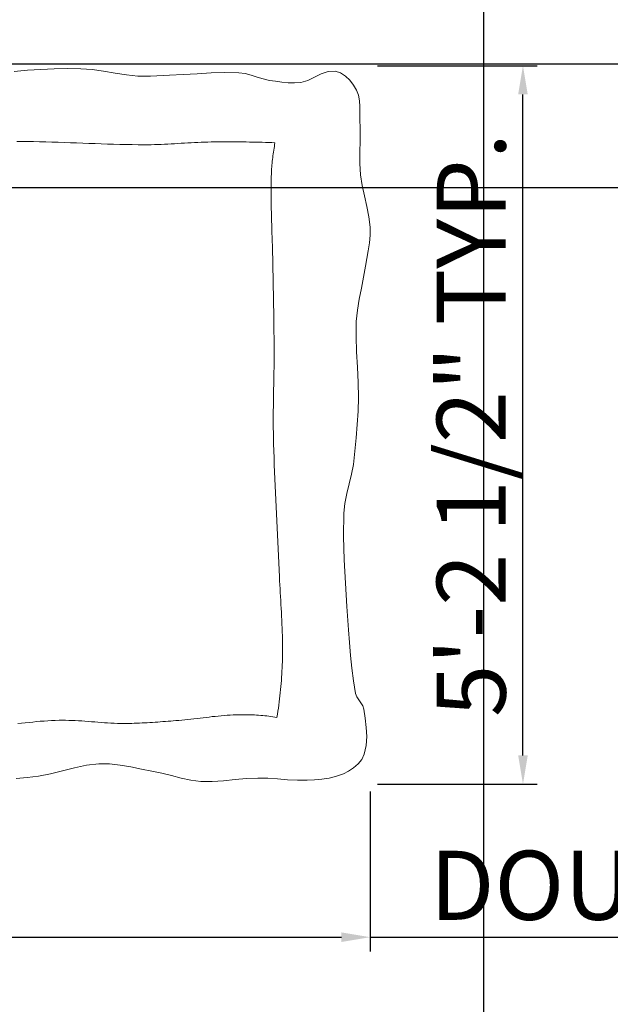
# Model space of a CAD drawing. Units: inches. Extents: x 2656 to 9931, y 1941 to 3068.
# Tile 12 of 46: x 2811 to 2863, y 2484 to 2569. Entities that reach past the tile are written whole.
import ezdxf

# ---------------------------------------------------------------- set-up
doc = ezdxf.new("R2010")
doc.units = ezdxf.units.IN
doc.layers.add('A-ANNO-DIMS', color=2, linetype='Continuous', lineweight=18)
doc.layers.add('A-FURN', color=8, linetype='Continuous', lineweight=13)
doc.styles.get("Standard").update_dxf_attribs({"font": 'arial.ttf'})
doc.dimstyles.new('ISO-25', dxfattribs={"dimtxt": 6, "dimasz": 2.5, "dimexe": 1.25, "dimexo": 0.625, "dimtad": 1, "dimdec": 0, "dimlunit": 3, "dimtxsty": 'Standard', "dimcen": 2.5, "dimadec": 0, "dimazin": 0, "dimtfac": 1, "dimtdec": 0, "dimtmove": 0, "dimatfit": 3, "dimfxl": 1, "dimarcsym": 0})

# ---------------------------------------------------------------- blocks, each defined once
blk = doc.blocks.new('BED-DOUBLE')
for p, q in [((58.764, 62.009), (57.607, 61.902)), ((59.923, 62.092), (58.764, 62.009)), ((61.084, 62.147), (59.923, 62.092)), ((62.246, 62.166), (61.084, 62.147)), ((63.407, 62.146), (62.246, 62.166)), ((64.403, 62.069), (63.407, 62.146)), ((65.395, 61.932), (64.403, 62.069)), ((66.384, 61.77), (65.395, 61.932)), ((67.375, 61.618), (66.384, 61.77)), ((68.37, 61.511), (67.375, 61.618)), ((72.325, 61.635), (71.116, 61.578)), ((73.533, 61.711), (72.325, 61.635)), ((74.742, 61.781), (73.533, 61.711)), ((75.95, 61.817), (74.742, 61.781)), ((77.158, 61.794), (75.95, 61.817)), ((77.698, 61.721), (77.158, 61.794)), ((78.229, 61.583), (77.698, 61.721)), ((84.331, 61.693), (83.743, 61.407)), ((84.926, 61.898), (84.331, 61.693)), ((85.537, 61.929), (84.926, 61.898)), ((86.008, 61.785), (85.537, 61.929)), ((86.434, 61.514), (86.008, 61.785)), ((68.918, 61.489), (68.37, 61.511)), ((69.467, 61.497), (68.918, 61.489)), ((70.017, 61.522), (69.467, 61.497)), ((70.567, 61.553), (70.017, 61.522)), ((71.116, 61.578), (70.567, 61.553)), ((78.755, 61.415), (78.229, 61.583)), ((79.283, 61.255), (78.755, 61.415)), ((79.819, 61.137), (79.283, 61.255)), ((80.36, 61.054), (79.819, 61.137)), ((80.905, 60.98), (80.36, 61.054)), ((81.45, 60.93), (80.905, 60.98)), ((81.996, 60.92), (81.45, 60.93)), ((82.537, 60.963), (81.996, 60.92)), ((83.149, 61.132), (82.537, 60.963)), ((83.743, 61.407), (83.149, 61.132)), ((86.811, 61.15), (86.434, 61.514)), ((87.134, 60.731), (86.811, 61.15)), ((87.398, 60.291), (87.134, 60.731)), ((87.572, 59.839), (87.398, 60.291)), ((87.658, 59.358), (87.572, 59.839)), ((87.686, 58.86), (87.658, 59.358)), ((87.688, 58.356), (87.686, 58.86)), ((87.698, 57.859), (87.688, 58.356)), ((87.718, 56.87), (87.698, 57.859)), ((87.706, 55.879), (87.718, 56.87)), ((58.21, 55.827), (57.849, 55.828)), ((58.746, 55.822), (58.21, 55.827)), ((59.283, 55.814), (58.746, 55.822)), ((59.819, 55.803), (59.283, 55.814)), ((60.355, 55.789), (59.819, 55.803)), ((60.892, 55.774), (60.355, 55.789)), ((61.428, 55.756), (60.892, 55.774)), ((61.964, 55.738), (61.428, 55.756)), ((62.5, 55.718), (61.964, 55.738)), ((63.037, 55.698), (62.5, 55.718)), ((63.573, 55.678), (63.037, 55.698)), ((64.109, 55.657), (63.573, 55.678)), ((64.645, 55.638), (64.109, 55.657)), ((65.181, 55.619), (64.645, 55.638)), ((65.718, 55.601), (65.181, 55.619)), ((71.546, 55.63), (71.256, 55.614)), ((71.836, 55.648), (71.546, 55.63)), ((72.126, 55.665), (71.836, 55.648)), ((72.416, 55.682), (72.126, 55.665)), ((72.706, 55.7), (72.416, 55.682)), ((72.996, 55.716), (72.706, 55.7)), ((73.286, 55.731), (72.996, 55.716)), ((73.576, 55.745), (73.286, 55.731)), ((73.866, 55.758), (73.576, 55.745)), ((74.156, 55.769), (73.866, 55.758)), ((74.446, 55.777), (74.156, 55.769)), ((74.736, 55.783), (74.446, 55.777)), ((75.014, 55.787), (74.736, 55.783)), ((75.293, 55.79), (75.014, 55.787)), ((75.571, 55.792), (75.293, 55.79)), ((75.85, 55.793), (75.571, 55.792)), ((76.128, 55.794), (75.85, 55.793)), ((76.406, 55.794), (76.128, 55.794)), ((76.685, 55.793), (76.406, 55.794)), ((76.963, 55.792), (76.685, 55.793)), ((77.242, 55.789), (76.963, 55.792)), ((77.52, 55.786), (77.242, 55.789)), ((77.799, 55.782), (77.52, 55.786)), ((78.077, 55.778), (77.799, 55.782)), ((78.355, 55.772), (78.077, 55.778)), ((78.634, 55.766), (78.355, 55.772)), ((78.912, 55.759), (78.634, 55.766)), ((79.19, 55.751), (78.912, 55.759)), ((79.469, 55.743), (79.19, 55.751)), ((79.747, 55.733), (79.469, 55.743)), ((80.025, 55.723), (79.747, 55.733)), ((80.303, 55.712), (80.025, 55.723)), ((80.274, 55.552), (80.303, 55.712)), ((87.688, 54.889), (87.706, 55.879)), ((66.254, 55.584), (65.718, 55.601)), ((66.79, 55.57), (66.254, 55.584)), ((67.327, 55.558), (66.79, 55.57)), ((67.863, 55.548), (67.327, 55.558)), ((68.399, 55.542), (67.863, 55.548)), ((68.936, 55.538), (68.399, 55.542)), ((69.226, 55.539), (68.936, 55.538)), ((69.516, 55.543), (69.226, 55.539)), ((69.806, 55.55), (69.516, 55.543)), ((70.096, 55.559), (69.806, 55.55)), ((70.386, 55.57), (70.096, 55.559)), ((70.676, 55.583), (70.386, 55.57)), ((70.966, 55.598), (70.676, 55.583)), ((71.256, 55.614), (70.966, 55.598)), ((80.146, 54.748), (80.169, 54.909)), ((80.169, 54.909), (80.193, 55.07)), ((80.193, 55.07), (80.219, 55.231)), ((80.219, 55.231), (80.246, 55.392)), ((80.246, 55.392), (80.274, 55.552)), ((87.693, 53.9), (87.688, 54.889)), ((80.038, 53.776), (80.053, 53.938)), ((80.053, 53.938), (80.069, 54.1)), ((80.069, 54.1), (80.086, 54.262)), ((80.086, 54.262), (80.105, 54.424)), ((80.105, 54.424), (80.125, 54.586)), ((80.125, 54.586), (80.146, 54.748)), ((79.985, 52.963), (79.993, 53.125)), ((79.993, 53.125), (80.002, 53.288)), ((80.002, 53.288), (80.013, 53.451)), ((80.013, 53.451), (80.025, 53.613)), ((80.025, 53.613), (80.038, 53.776)), ((87.749, 52.913), (87.693, 53.9)), ((79.965, 52.119), (79.97, 52.475)), ((79.97, 52.475), (79.974, 52.637)), ((79.974, 52.637), (79.979, 52.8)), ((79.979, 52.8), (79.985, 52.963)), ((87.883, 51.998), (87.749, 52.913)), ((79.962, 51.764), (79.965, 52.119)), ((79.962, 51.408), (79.962, 51.764)), ((79.963, 51.053), (79.962, 51.408)), ((88.08, 51.092), (87.883, 51.998)), ((79.967, 50.698), (79.963, 51.053)), ((79.972, 50.342), (79.967, 50.698)), ((88.293, 50.188), (88.08, 51.092)), ((79.979, 49.987), (79.972, 50.342)), ((79.988, 49.631), (79.979, 49.987)), ((79.997, 49.276), (79.988, 49.631)), ((88.476, 49.281), (88.293, 50.188)), ((80.007, 48.921), (79.997, 49.276)), ((80.018, 48.565), (80.007, 48.921)), ((88.582, 48.364), (88.476, 49.281)), ((80.029, 48.21), (80.018, 48.565)), ((80.041, 47.854), (80.029, 48.21)), ((88.58, 47.686), (88.582, 48.364)), ((80.052, 47.499), (80.041, 47.854)), ((80.063, 47.143), (80.052, 47.499)), ((80.074, 46.788), (80.063, 47.143)), ((88.516, 47.01), (88.58, 47.686)), ((80.084, 46.433), (80.074, 46.788)), ((80.094, 46.077), (80.084, 46.433)), ((88.294, 45.661), (88.413, 46.334)), ((88.413, 46.334), (88.516, 47.01)), ((80.102, 45.722), (80.094, 46.077)), ((80.109, 45.366), (80.102, 45.722)), ((80.115, 44.982), (80.109, 45.366)), ((88.183, 44.988), (88.294, 45.661)), ((80.123, 44.597), (80.115, 44.982)), ((80.13, 44.212), (80.123, 44.597)), ((88.016, 44.028), (88.183, 44.988)), ((80.137, 43.828), (80.13, 44.212)), ((80.145, 43.443), (80.137, 43.828)), ((87.82, 43.073), (88.016, 44.028)), ((80.152, 43.059), (80.145, 43.443)), ((80.159, 42.674), (80.152, 43.059)), ((87.627, 42.118), (87.82, 43.073)), ((80.167, 42.289), (80.159, 42.674)), ((80.174, 41.905), (80.167, 42.289)), ((87.467, 41.159), (87.627, 42.118)), ((80.181, 41.52), (80.174, 41.905)), ((80.188, 41.135), (80.181, 41.52)), ((80.194, 40.751), (80.188, 41.135)), ((87.372, 40.192), (87.467, 41.159)), ((80.2, 40.366), (80.194, 40.751)), ((80.206, 39.982), (80.2, 40.366)), ((80.211, 39.597), (80.206, 39.982)), ((80.215, 39.212), (80.211, 39.597)), ((87.351, 38.868), (87.372, 40.192)), ((80.219, 38.828), (80.215, 39.212)), ((80.223, 38.443), (80.219, 38.828)), ((87.402, 37.543), (87.351, 38.868)), ((80.225, 38.058), (80.223, 38.443)), ((80.227, 37.674), (80.225, 38.058)), ((80.228, 37.297), (80.227, 37.674)), ((80.224, 36.545), (80.226, 36.921)), ((80.226, 36.921), (80.228, 37.297)), ((87.483, 36.218), (87.402, 37.543)), ((80.214, 35.792), (80.22, 36.168)), ((80.22, 36.168), (80.224, 36.545)), ((87.553, 34.892), (87.483, 36.218)), ((80.202, 35.04), (80.208, 35.416)), ((80.208, 35.416), (80.214, 35.792)), ((80.18, 33.911), (80.187, 34.287)), ((80.187, 34.287), (80.195, 34.663)), ((80.195, 34.663), (80.202, 35.04)), ((87.568, 33.566), (87.553, 34.892)), ((80.168, 33.158), (80.174, 33.534)), ((80.174, 33.534), (80.18, 33.911)), ((87.531, 32.4), (87.568, 33.566)), ((80.158, 32.406), (80.162, 32.782)), ((80.162, 32.782), (80.168, 33.158)), ((80.154, 31.653), (80.156, 32.029)), ((80.156, 32.029), (80.158, 32.406)), ((87.466, 31.235), (87.531, 32.4)), ((80.155, 31.277), (80.154, 31.653)), ((80.158, 30.901), (80.155, 31.277)), ((80.162, 30.524), (80.158, 30.901)), ((87.376, 30.07), (87.466, 31.235)), ((80.17, 30.148), (80.162, 30.524)), ((80.185, 29.54), (80.17, 30.148)), ((87.262, 28.909), (87.376, 30.07)), ((80.203, 28.931), (80.185, 29.54)), ((80.223, 28.323), (80.203, 28.931)), ((80.244, 27.714), (80.223, 28.323)), ((87.125, 27.75), (87.262, 28.909)), ((80.268, 27.106), (80.244, 27.714)), ((86.972, 26.9), (87.125, 27.75)), ((80.292, 26.497), (80.268, 27.106)), ((86.762, 26.059), (86.972, 26.9)), ((80.318, 25.889), (80.292, 26.497)), ((80.346, 25.281), (80.318, 25.889)), ((86.546, 25.219), (86.762, 26.059)), ((80.374, 24.672), (80.346, 25.281)), ((86.37, 24.375), (86.546, 25.219)), ((80.402, 24.064), (80.374, 24.672)), ((80.432, 23.456), (80.402, 24.064)), ((86.283, 23.521), (86.37, 24.375)), ((80.461, 22.848), (80.432, 23.456)), ((86.267, 21.495), (86.283, 23.521)), ((80.491, 22.24), (80.461, 22.848)), ((80.521, 21.631), (80.491, 22.24)), ((80.551, 21.023), (80.521, 21.631)), ((86.324, 19.469), (86.267, 21.495)), ((80.58, 20.415), (80.551, 21.023)), ((80.609, 19.807), (80.58, 20.415)), ((80.637, 19.198), (80.609, 19.807)), ((80.664, 18.59), (80.637, 19.198)), ((86.43, 17.443), (86.324, 19.469)), ((80.69, 17.982), (80.664, 18.59)), ((80.705, 17.64), (80.69, 17.982)), ((80.721, 17.299), (80.705, 17.64)), ((80.739, 16.957), (80.721, 17.299)), ((86.563, 15.419), (86.43, 17.443)), ((80.758, 16.616), (80.739, 16.957)), ((80.777, 16.275), (80.758, 16.616)), ((80.797, 15.933), (80.777, 16.275)), ((80.817, 15.592), (80.797, 15.933)), ((80.837, 15.25), (80.817, 15.592)), ((86.702, 13.396), (86.563, 15.419)), ((80.856, 14.909), (80.837, 15.25)), ((80.875, 14.567), (80.856, 14.909)), ((80.893, 14.226), (80.875, 14.567)), ((80.909, 13.884), (80.893, 14.226)), ((80.924, 13.543), (80.909, 13.884)), ((80.937, 13.201), (80.924, 13.543)), ((80.947, 12.86), (80.937, 13.201)), ((80.956, 12.518), (80.947, 12.86)), ((86.779, 12.281), (86.702, 13.396)), ((80.961, 12.177), (80.956, 12.518)), ((80.964, 11.835), (80.961, 12.177)), ((86.87, 11.166), (86.779, 12.281)), ((80.953, 10.882), (80.959, 11.152)), ((80.959, 11.152), (80.963, 11.493)), ((80.963, 11.493), (80.964, 11.835)), ((86.984, 10.054), (86.87, 11.166)), ((80.924, 10.073), (80.936, 10.343)), ((80.936, 10.343), (80.945, 10.612)), ((80.945, 10.612), (80.953, 10.882)), ((80.877, 9.265), (80.895, 9.534)), ((80.895, 9.534), (80.91, 9.804)), ((80.91, 9.804), (80.924, 10.073)), ((87.13, 8.946), (86.984, 10.054)), ((80.813, 8.457), (80.836, 8.726)), ((80.836, 8.726), (80.858, 8.995)), ((80.858, 8.995), (80.877, 9.265)), ((87.318, 7.845), (87.13, 8.946)), ((80.731, 7.651), (80.76, 7.92)), ((80.76, 7.92), (80.787, 8.188)), ((80.787, 8.188), (80.813, 8.457)), ((87.423, 7.56), (87.318, 7.845)), ((80.594, 6.58), (80.631, 6.848)), ((80.631, 6.848), (80.666, 7.115)), ((80.666, 7.115), (80.699, 7.383)), ((80.699, 7.383), (80.731, 7.651)), ((87.593, 7.296), (87.423, 7.56)), ((87.782, 7.04), (87.593, 7.296)), ((87.945, 6.776), (87.782, 7.04)), ((76.401, 5.979), (76.664, 5.993)), ((76.664, 5.993), (76.927, 6.003)), ((76.927, 6.003), (77.105, 6.008)), ((77.105, 6.008), (77.282, 6.011)), ((77.282, 6.011), (77.46, 6.013)), ((77.46, 6.013), (77.638, 6.012)), ((77.638, 6.012), (77.816, 6.011)), ((77.816, 6.011), (77.994, 6.007)), ((77.994, 6.007), (78.171, 6.002)), ((78.171, 6.002), (78.349, 5.995)), ((78.349, 5.995), (78.527, 5.986)), ((80.471, 5.78), (80.514, 6.047)), ((80.514, 6.047), (80.555, 6.313)), ((80.555, 6.313), (80.594, 6.58)), ((88.038, 6.488), (87.945, 6.776)), ((88.149, 5.704), (88.038, 6.488)), ((57.93, 5.241), (58.256, 5.275)), ((58.256, 5.275), (58.581, 5.31)), ((58.581, 5.31), (58.906, 5.343)), ((58.906, 5.343), (59.232, 5.376)), ((59.232, 5.376), (59.557, 5.407)), ((59.557, 5.407), (59.883, 5.436)), ((59.883, 5.436), (60.208, 5.461)), ((60.208, 5.461), (60.534, 5.484)), ((60.534, 5.484), (60.86, 5.502)), ((60.86, 5.502), (61.187, 5.516)), ((61.187, 5.516), (61.513, 5.525)), ((61.513, 5.525), (61.796, 5.528)), ((61.796, 5.528), (62.078, 5.526)), ((62.078, 5.526), (62.36, 5.52)), ((62.36, 5.52), (62.642, 5.51)), ((62.642, 5.51), (62.924, 5.497)), ((62.924, 5.497), (63.206, 5.482)), ((63.206, 5.482), (63.488, 5.464)), ((63.488, 5.464), (63.77, 5.445)), ((63.77, 5.445), (64.052, 5.424)), ((64.052, 5.424), (64.334, 5.402)), ((64.334, 5.402), (64.616, 5.381)), ((64.616, 5.381), (64.897, 5.359)), ((64.897, 5.359), (65.179, 5.338)), ((65.179, 5.338), (65.461, 5.318)), ((65.461, 5.318), (65.743, 5.3)), ((65.743, 5.3), (66.025, 5.284)), ((66.025, 5.284), (66.307, 5.27)), ((66.307, 5.27), (66.59, 5.26)), ((66.59, 5.26), (66.872, 5.253)), ((66.872, 5.253), (67.154, 5.25)), ((67.154, 5.25), (67.381, 5.25)), ((67.381, 5.25), (67.608, 5.253)), ((67.608, 5.253), (67.834, 5.257)), ((67.834, 5.257), (68.061, 5.263)), ((68.061, 5.263), (68.288, 5.271)), ((68.288, 5.271), (68.514, 5.28)), ((68.514, 5.28), (68.741, 5.29)), ((68.741, 5.29), (68.967, 5.302)), ((68.967, 5.302), (69.194, 5.315)), ((69.194, 5.315), (69.42, 5.329)), ((69.42, 5.329), (69.647, 5.343)), ((69.647, 5.343), (69.873, 5.359)), ((69.873, 5.359), (70.1, 5.375)), ((70.1, 5.375), (70.326, 5.392)), ((70.326, 5.392), (70.552, 5.409)), ((70.552, 5.409), (70.778, 5.427)), ((70.778, 5.427), (71.005, 5.445)), ((71.005, 5.445), (71.231, 5.462)), ((71.231, 5.462), (71.457, 5.48)), ((71.457, 5.48), (71.683, 5.498)), ((71.683, 5.498), (71.946, 5.519)), ((71.946, 5.519), (72.208, 5.543)), ((72.208, 5.543), (72.47, 5.569)), ((72.47, 5.569), (72.732, 5.597)), ((72.732, 5.597), (72.994, 5.626)), ((72.994, 5.626), (73.256, 5.656)), ((73.256, 5.656), (73.518, 5.686)), ((73.518, 5.686), (73.78, 5.718)), ((73.78, 5.718), (74.042, 5.749)), ((74.042, 5.749), (74.304, 5.78)), ((74.304, 5.78), (74.565, 5.81)), ((74.565, 5.81), (74.827, 5.84)), ((74.827, 5.84), (75.089, 5.868)), ((75.089, 5.868), (75.351, 5.895)), ((75.351, 5.895), (75.614, 5.919)), ((75.614, 5.919), (75.876, 5.942)), ((75.876, 5.942), (76.138, 5.962)), ((76.138, 5.962), (76.401, 5.979)), ((78.527, 5.986), (78.705, 5.976)), ((78.705, 5.976), (78.882, 5.964)), ((78.882, 5.964), (79.06, 5.95)), ((79.06, 5.95), (79.237, 5.935)), ((79.237, 5.935), (79.414, 5.918)), ((79.414, 5.918), (79.591, 5.899)), ((79.591, 5.899), (79.767, 5.879)), ((79.767, 5.879), (79.944, 5.856)), ((79.944, 5.856), (80.12, 5.833)), ((80.12, 5.833), (80.296, 5.807)), ((80.296, 5.807), (80.471, 5.78)), ((88.241, 4.91), (88.149, 5.704)), ((88.279, 4.116), (88.241, 4.91)), ((88.232, 3.333), (88.279, 4.116)), ((87.852, 2.127), (88.065, 2.573)), ((88.065, 2.573), (88.232, 3.333)), ((63.916, 1.633), (64.981, 1.753)), ((64.981, 1.753), (65.91, 1.738)), ((65.91, 1.738), (66.836, 1.633)), ((87.142, 1.396), (87.535, 1.735)), ((87.535, 1.735), (87.852, 2.127)), ((59.716, 0.663), (60.773, 0.866)), ((60.773, 0.866), (61.82, 1.133)), ((61.82, 1.133), (62.865, 1.407)), ((62.865, 1.407), (63.916, 1.633)), ((66.836, 1.633), (67.759, 1.471)), ((67.759, 1.471), (68.68, 1.285)), ((68.68, 1.285), (69.6, 1.109)), ((69.6, 1.109), (70.45, 0.931)), ((70.45, 0.931), (71.295, 0.716)), ((85.653, 0.657), (86.251, 0.879)), ((86.251, 0.879), (86.705, 1.111)), ((86.705, 1.111), (87.142, 1.396)), ((57.788, 0.467), (58.754, 0.547)), ((58.754, 0.547), (59.716, 0.663)), ((71.295, 0.716), (72.139, 0.5)), ((72.139, 0.5), (72.988, 0.322)), ((72.988, 0.322), (73.847, 0.217)), ((73.847, 0.217), (74.842, 0.204)), ((74.842, 0.204), (75.836, 0.268)), ((75.836, 0.268), (76.831, 0.367)), ((76.831, 0.367), (77.826, 0.461)), ((77.826, 0.461), (78.822, 0.509)), ((78.822, 0.509), (79.679, 0.489)), ((79.679, 0.489), (80.535, 0.43)), ((80.535, 0.43), (81.391, 0.362)), ((81.391, 0.362), (82.248, 0.316)), ((82.248, 0.316), (83.104, 0.322)), ((83.104, 0.322), (83.746, 0.358)), ((83.746, 0.358), (84.392, 0.414)), ((84.392, 0.414), (85.03, 0.508)), ((85.03, 0.508), (85.653, 0.657))]:
    blk.add_line(p, q)
blk = doc.blocks.new('*D31')
at = {"layer": 'A-ANNO-DIMS', "color": 0, "lineweight": -2, "transparency": 16777216}
for p, q in [((2753.358, 2502.145), (2753.358, 2488.227)), ((2841.982, 2502.145), (2841.982, 2488.227)), ((2755.858, 2489.477), (2839.482, 2489.477)), ((2841.982, 2489.477), (2952.348, 2489.477))]:
    blk.add_line(p, q, dxfattribs=at)
at = {"layer": 'A-ANNO-DIMS', "color": 0, "transparency": 16777216}
for points in [[(2755.858, 2489.893), (2755.858, 2489.06), (2753.358, 2489.477)], [(2839.482, 2489.893), (2839.482, 2489.06), (2841.982, 2489.477)]]:
    blk.add_solid(points, dxfattribs=at)
at = {"layer": 'Defpoints', "color": 0, "transparency": 16777216}
for p in [(2753.358, 2502.77), (2841.982, 2502.77), (2841.982, 2489.477)]:
    blk.add_point(p, dxfattribs=at)
at = {"layer": 'A-ANNO-DIMS', "color": 0, "transparency": 16777216, "insert": (2898.415, 2493.206), "char_height": 6, "attachment_point": 5}
blk.add_mtext('DOUBLE BED 7\'-4 1/2" TYP.', dxfattribs=at)
blk = doc.blocks.new('*D32')
at = {"layer": 'A-ANNO-DIMS', "color": 0, "lineweight": -2, "transparency": 16777216}
for p, q in [((2842.607, 2565.211), (2856.525, 2565.211)), ((2855.275, 2505.27), (2855.275, 2562.711)), ((2842.607, 2502.77), (2856.525, 2502.77))]:
    blk.add_line(p, q, dxfattribs=at)
at = {"layer": 'A-ANNO-DIMS', "color": 0, "transparency": 16777216}
for points in [[(2854.858, 2562.711), (2855.692, 2562.711), (2855.275, 2565.211)], [(2854.858, 2505.27), (2855.692, 2505.27), (2855.275, 2502.77)]]:
    blk.add_solid(points, dxfattribs=at)
at = {"layer": 'Defpoints', "color": 0, "transparency": 16777216}
for p in [(2841.982, 2565.211), (2855.275, 2565.211), (2841.982, 2502.77)]:
    blk.add_point(p, dxfattribs=at)
at = {"layer": 'A-ANNO-DIMS', "color": 0, "transparency": 16777216, "insert": (2851.548, 2533.991), "char_height": 6, "attachment_point": 5, "rotation": 90}
blk.add_mtext('5\'-2 1/2" TYP.', dxfattribs=at)
blk = doc.blocks.new('*D100')
at = {"layer": 'A-ANNO-DIMS', "color": 0, "lineweight": -2, "transparency": 16777216}
for p, q in [((2696.557, 2565.337), (2696.557, 2603.679)), ((2876.032, 2565.337), (2695.307, 2565.337)), ((2696.557, 2557.1), (2696.557, 2562.837)), ((2876.032, 2554.6), (2695.307, 2554.6))]:
    blk.add_line(p, q, dxfattribs=at)
at = {"layer": 'A-ANNO-DIMS', "color": 0, "transparency": 16777216}
for points in [[(2696.141, 2562.837), (2696.974, 2562.837), (2696.557, 2565.337)], [(2696.141, 2557.1), (2696.974, 2557.1), (2696.557, 2554.6)]]:
    blk.add_solid(points, dxfattribs=at)
at = {"layer": 'Defpoints', "color": 0, "transparency": 16777216}
for p in [(2696.557, 2565.337), (2876.657, 2565.337), (2876.657, 2554.6)]:
    blk.add_point(p, dxfattribs=at)
at = {"layer": 'A-ANNO-DIMS', "color": 0, "transparency": 16777216, "insert": (2692.83, 2585.758), "char_height": 6, "attachment_point": 5, "rotation": 90}
blk.add_mtext('0\'-10 1/2"', dxfattribs=at)
blk = doc.blocks.new('*D114')
at = {"layer": 'A-ANNO-DIMS', "color": 0, "lineweight": -2, "transparency": 16777216}
for p, q in [((2809.769, 2300.725), (2809.769, 2674.45)), ((2851.877, 2300.725), (2851.877, 2674.45)), ((2812.269, 2673.2), (2849.377, 2673.2))]:
    blk.add_line(p, q, dxfattribs=at)
at = {"layer": 'A-ANNO-DIMS', "color": 0, "transparency": 16777216}
for points in [[(2812.269, 2673.617), (2812.269, 2672.784), (2809.769, 2673.2)], [(2849.377, 2673.617), (2849.377, 2672.784), (2851.877, 2673.2)]]:
    blk.add_solid(points, dxfattribs=at)
at = {"layer": 'Defpoints', "color": 0, "transparency": 16777216}
for p in [(2851.877, 2673.2), (2809.769, 2300.1), (2851.877, 2300.1)]:
    blk.add_point(p, dxfattribs=at)
at = {"layer": 'A-ANNO-DIMS', "color": 0, "transparency": 16777216, "insert": (2830.823, 2676.891), "char_height": 6, "attachment_point": 5}
blk.add_mtext('3\'-6"', dxfattribs=at)
blk = doc.blocks.new('*D137')
at = {"layer": 'A-ANNO-DIMS', "color": 0, "lineweight": -2, "transparency": 16777216}
for p, q in [((2779.142, 2375.042), (2779.142, 2674.45)), ((2792.516, 2375.042), (2792.516, 2674.45)), ((2781.642, 2673.2), (2790.016, 2673.2)), ((2792.516, 2673.2), (2825.632, 2673.2))]:
    blk.add_line(p, q, dxfattribs=at)
at = {"layer": 'A-ANNO-DIMS', "color": 0, "transparency": 16777216}
for points in [[(2781.642, 2673.617), (2781.642, 2672.784), (2779.142, 2673.2)], [(2790.016, 2673.617), (2790.016, 2672.784), (2792.516, 2673.2)]]:
    blk.add_solid(points, dxfattribs=at)
at = {"layer": 'Defpoints', "color": 0, "transparency": 16777216}
for p in [(2792.516, 2673.2), (2779.142, 2374.417), (2792.516, 2374.417)]:
    blk.add_point(p, dxfattribs=at)
at = {"layer": 'A-ANNO-DIMS', "color": 0, "transparency": 16777216, "insert": (2810.324, 2676.928), "char_height": 6, "attachment_point": 5}
blk.add_mtext('1\'-1 1/2"', dxfattribs=at)

msp = doc.modelspace()

# ---------------------------------------------------------------- block references
at = {"layer": 'A-FURN'}
msp.add_blockref('BED-DOUBLE', (2753.4, 2502.8), dxfattribs=at)

# ---------------------------------------------------------------- dimensions: what is measured, and where the dimension line sits
at = {"layer": 'A-ANNO-DIMS'}
for base, p1, p2, picture, middle in [((2792.516, 2673.2), (2779.142, 2374.417), (2792.516, 2374.417), '*D137', (2810.324, 2676.928)), ((2851.877, 2673.2), (2809.769, 2300.1), (2851.877, 2300.1), '*D114', (2830.823, 2676.891))]:
    dim = msp.add_linear_dim(base=base, p1=p1, p2=p2, dimstyle='ISO-25', override={"dimdec": 1, "dimlfac": 1, "dimrnd": 0, "dimzin": 1, "dimdsep": 46, "dimlunit": 4, "dimfrac": 2}, dxfattribs=at)
    dim.commit()
    dim.dimension.update_dxf_attribs({"geometry": picture, "text_midpoint": middle})
dim = msp.add_linear_dim(base=(2696.557, 2565.337), p1=(2876.657, 2554.6), p2=(2876.657, 2565.337), angle=90, dimstyle='ISO-25', override={"dimdec": 1, "dimlfac": 1, "dimrnd": 0, "dimzin": 1, "dimdsep": 46, "dimlunit": 4, "dimfrac": 2}, dxfattribs=at)
dim.commit()
dim.dimension.update_dxf_attribs({"geometry": '*D100', "text_midpoint": (2692.83, 2585.758)})
dim = msp.add_linear_dim(base=(2855.275, 2565.211), p1=(2841.982, 2502.77), p2=(2841.982, 2565.211), angle=90, text='<> TYP.', dimstyle='ISO-25', override={"dimdec": 1, "dimlfac": 1, "dimrnd": 0, "dimzin": 1, "dimdsep": 46, "dimlunit": 4, "dimfrac": 2}, dxfattribs=at)
dim.commit()
dim.dimension.update_dxf_attribs({"geometry": '*D32', "text_midpoint": (2851.548, 2533.991)})
dim = msp.add_linear_dim(base=(2841.982, 2489.477), p1=(2753.358, 2502.77), p2=(2841.982, 2502.77), text='DOUBLE BED <> TYP.', dimstyle='ISO-25', override={"dimdec": 1, "dimlfac": 1, "dimrnd": 0, "dimzin": 1, "dimdsep": 46, "dimlunit": 4, "dimfrac": 2}, dxfattribs=at)
dim.commit()
dim.dimension.update_dxf_attribs({"geometry": '*D31', "text_midpoint": (2898.415, 2493.206)})

doc.saveas('drawing.dxf')
